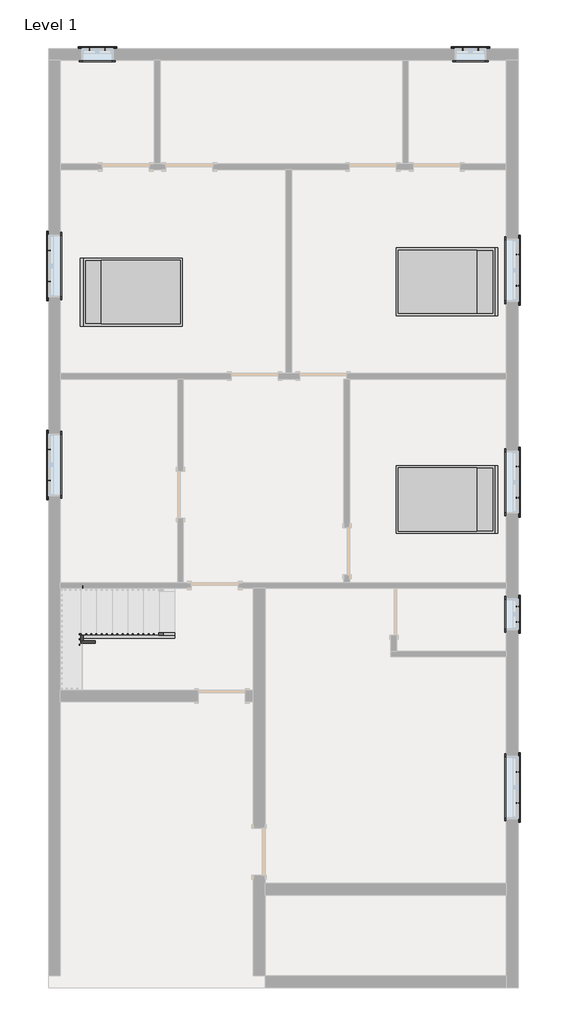
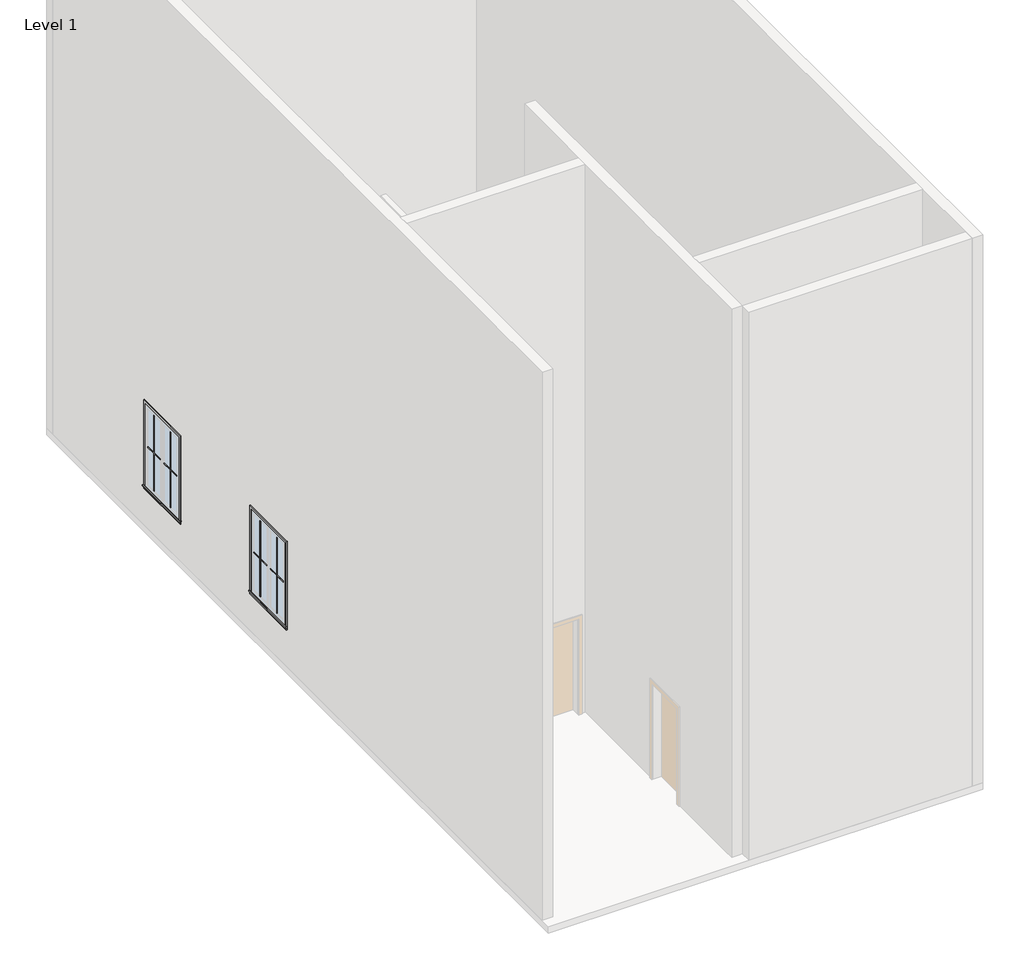
# One storey, part 2 of 2: 32 proxies, 6 members, 3 furniture elements, 1 railing.
"""IFC4 building model written with IfcOpenShell, lengths in millimetres."""

from ifc_helpers import new_model, si_unit, frame, origin, place, context, project, spatial, polyline, outline, extrude, faceted_brep, transform, mapped, element, save
from components import muntin_pattern_2x2_muntin_pattern_2x2_2b4d9f72, muntin_pattern_2x2_muntin_pattern_2x2_ef995ed3, muntin_pattern_2x2_muntin_pattern_2x2_53152e2c, muntin_pattern_2x2_muntin_pattern_2x2_e8f3e573, trim_window_exterior_flat_with_sill_b7e4d11c, trim_window_exterior_flat_with_sill_a665a915, trim_window_interior_flat_picture_frame_936b8d2a, trim_window_interior_flat_picture_frame_d485c387, bed_17739_bed_17739_15c61121

model = new_model("IFC4")

# Units and contexts
model_context = context("Model", 3, world=origin())
ifc_project = project(units=[si_unit("LENGTHUNIT", "METRE", prefix="MILLI")], contexts=[model_context])

# Site, building, storey
site = spatial("IfcSite", under=ifc_project)
building = spatial("IfcBuilding", under=site)
storey = spatial("IfcBuildingStorey", under=building, Name="Level 1", Elevation=0.0)

# Proxies
placement = place(None, origin())
muntin_pattern_2x2_muntin_pattern_2x2_shape = muntin_pattern_2x2_muntin_pattern_2x2_2b4d9f72(model_context)
element("IfcBuildingElementProxy", 1, Name="Muntin Pattern_2x2 : Muntin Pattern_2x2", ObjectType="Muntin Pattern_2x2 : Muntin Pattern_2x2", at=placement, inside=storey, context=model_context, shape_type="MappedRepresentation", body=[
    mapped(muntin_pattern_2x2_muntin_pattern_2x2_shape, transform((1279.525, 5811.8375, 984.25), x_axis=(0.0, 1.0, 0.0), y_axis=(-1.0, 0.0, 0.0), z_axis=(0.0, 0.0, 1.0))),
])
element("IfcBuildingElementProxy", 2, Name="Muntin Pattern_2x2 : Muntin Pattern_2x2", ObjectType="Muntin Pattern_2x2 : Muntin Pattern_2x2", at=placement, inside=storey, context=model_context, shape_type="MappedRepresentation", body=[
    mapped(muntin_pattern_2x2_muntin_pattern_2x2_shape, transform((1279.525, 9685.3375, 984.25), x_axis=(0.0, 1.0, 0.0), y_axis=(-1.0, 0.0, 0.0), z_axis=(0.0, 0.0, 1.0))),
])
element("IfcBuildingElementProxy", 3, Name="Muntin Pattern_2x2 : Muntin Pattern_2x2", ObjectType="Muntin Pattern_2x2 : Muntin Pattern_2x2", at=placement, inside=storey, context=model_context, shape_type="MappedRepresentation", body=[
    mapped(muntin_pattern_2x2_muntin_pattern_2x2_shape, transform((10404.475, 10209.2125, 984.25), x_axis=(0.0, -1.0, 0.0), y_axis=(1.0, 0.0, 0.0), z_axis=(0.0, 0.0, 1.0))),
])
element("IfcBuildingElementProxy", 4, Name="Muntin Pattern_2x2 : Muntin Pattern_2x2", ObjectType="Muntin Pattern_2x2 : Muntin Pattern_2x2", at=placement, inside=storey, context=model_context, shape_type="MappedRepresentation", body=[
    mapped(muntin_pattern_2x2_muntin_pattern_2x2_shape, transform((10404.475, 6081.7125, 984.25), x_axis=(0.0, -1.0, 0.0), y_axis=(1.0, 0.0, 0.0), z_axis=(0.0, 0.0, 1.0))),
])
element("IfcBuildingElementProxy", 5, Name="Muntin Pattern_2x2 : Muntin Pattern_2x2", ObjectType="Muntin Pattern_2x2 : Muntin Pattern_2x2", at=placement, inside=storey, context=model_context, shape_type="MappedRepresentation", body=[
    mapped(muntin_pattern_2x2_muntin_pattern_2x2_shape, transform((10404.475, 138.1125, 984.25), x_axis=(0.0, -1.0, 0.0), y_axis=(1.0, 0.0, 0.0), z_axis=(0.0, 0.0, 1.0))),
])
muntin_pattern_2x2_muntin_pattern_2x2_2_shape = muntin_pattern_2x2_muntin_pattern_2x2_ef995ed3(model_context)
element("IfcBuildingElementProxy", 6, Name="Muntin Pattern_2x2 : Muntin Pattern_2x2", ObjectType="Muntin Pattern_2x2 : Muntin Pattern_2x2", at=placement, inside=storey, context=model_context, shape_type="MappedRepresentation", body=[
    mapped(muntin_pattern_2x2_muntin_pattern_2x2_2_shape, transform((1279.525, 6418.2625, 984.25), x_axis=(0.0, -1.0, 0.0), y_axis=(1.0, 0.0, 0.0), z_axis=(0.0, 0.0, 1.0))),
])
element("IfcBuildingElementProxy", 7, Name="Muntin Pattern_2x2 : Muntin Pattern_2x2", ObjectType="Muntin Pattern_2x2 : Muntin Pattern_2x2", at=placement, inside=storey, context=model_context, shape_type="MappedRepresentation", body=[
    mapped(muntin_pattern_2x2_muntin_pattern_2x2_2_shape, transform((1279.525, 10291.7625, 984.25), x_axis=(0.0, -1.0, 0.0), y_axis=(1.0, 0.0, 0.0), z_axis=(0.0, 0.0, 1.0))),
])
element("IfcBuildingElementProxy", 8, Name="Muntin Pattern_2x2 : Muntin Pattern_2x2", ObjectType="Muntin Pattern_2x2 : Muntin Pattern_2x2", at=placement, inside=storey, context=model_context, shape_type="MappedRepresentation", body=[
    mapped(muntin_pattern_2x2_muntin_pattern_2x2_2_shape, transform((10404.475, 9602.7875, 984.25), x_axis=(0.0, 1.0, 0.0), y_axis=(-1.0, 0.0, 0.0), z_axis=(0.0, 0.0, 1.0))),
])
element("IfcBuildingElementProxy", 9, Name="Muntin Pattern_2x2 : Muntin Pattern_2x2", ObjectType="Muntin Pattern_2x2 : Muntin Pattern_2x2", at=placement, inside=storey, context=model_context, shape_type="MappedRepresentation", body=[
    mapped(muntin_pattern_2x2_muntin_pattern_2x2_2_shape, transform((10404.475, 5475.2875, 984.25), x_axis=(0.0, 1.0, 0.0), y_axis=(-1.0, 0.0, 0.0), z_axis=(0.0, 0.0, 1.0))),
])
element("IfcBuildingElementProxy", 10, Name="Muntin Pattern_2x2 : Muntin Pattern_2x2", ObjectType="Muntin Pattern_2x2 : Muntin Pattern_2x2", at=placement, inside=storey, context=model_context, shape_type="MappedRepresentation", body=[
    mapped(muntin_pattern_2x2_muntin_pattern_2x2_2_shape, transform((10404.475, -468.3125, 984.25), x_axis=(0.0, 1.0, 0.0), y_axis=(-1.0, 0.0, 0.0), z_axis=(0.0, 0.0, 1.0))),
])
muntin_pattern_2x2_muntin_pattern_2x2_3_shape = muntin_pattern_2x2_muntin_pattern_2x2_53152e2c(model_context)
element("IfcBuildingElementProxy", 11, Name="Muntin Pattern_2x2 : Muntin Pattern_2x2", ObjectType="Muntin Pattern_2x2 : Muntin Pattern_2x2", at=placement, inside=storey, context=model_context, shape_type="MappedRepresentation", body=[
    mapped(muntin_pattern_2x2_muntin_pattern_2x2_3_shape, transform((10404.475, 3357.5625, 984.25), x_axis=(0.0, -1.0, 0.0), y_axis=(1.0, 0.0, 0.0), z_axis=(0.0, 0.0, 1.0))),
])
element("IfcBuildingElementProxy", 12, Name="Muntin Pattern_2x2 : Muntin Pattern_2x2", ObjectType="Muntin Pattern_2x2 : Muntin Pattern_2x2", at=placement, inside=storey, context=model_context, shape_type="MappedRepresentation", body=[
    mapped(muntin_pattern_2x2_muntin_pattern_2x2_3_shape, transform((9336.0875, 14214.475, 984.25), x_axis=(1.0, 0.0, 0.0), y_axis=(0.0, 1.0, 0.0), z_axis=(0.0, 0.0, 1.0))),
])
element("IfcBuildingElementProxy", 13, Name="Muntin Pattern_2x2 : Muntin Pattern_2x2", ObjectType="Muntin Pattern_2x2 : Muntin Pattern_2x2", at=placement, inside=storey, context=model_context, shape_type="MappedRepresentation", body=[
    mapped(muntin_pattern_2x2_muntin_pattern_2x2_3_shape, transform((2071.6875, 14214.475, 984.25), x_axis=(1.0, 0.0, 0.0), y_axis=(0.0, 1.0, 0.0), z_axis=(0.0, 0.0, 1.0))),
])
muntin_pattern_2x2_muntin_pattern_2x2_4_shape = muntin_pattern_2x2_muntin_pattern_2x2_e8f3e573(model_context)
element("IfcBuildingElementProxy", 14, Name="Muntin Pattern_2x2 : Muntin Pattern_2x2", ObjectType="Muntin Pattern_2x2 : Muntin Pattern_2x2", at=placement, inside=storey, context=model_context, shape_type="MappedRepresentation", body=[
    mapped(muntin_pattern_2x2_muntin_pattern_2x2_4_shape, transform((10404.475, 3055.9375, 984.25), x_axis=(0.0, 1.0, 0.0), y_axis=(-1.0, 0.0, 0.0), z_axis=(0.0, 0.0, 1.0))),
])
element("IfcBuildingElementProxy", 15, Name="Muntin Pattern_2x2 : Muntin Pattern_2x2", ObjectType="Muntin Pattern_2x2 : Muntin Pattern_2x2", at=placement, inside=storey, context=model_context, shape_type="MappedRepresentation", body=[
    mapped(muntin_pattern_2x2_muntin_pattern_2x2_4_shape, transform((9637.7125, 14214.475, 984.25), x_axis=(-1.0, 0.0, 0.0), y_axis=(0.0, -1.0, 0.0), z_axis=(0.0, 0.0, 1.0))),
])
element("IfcBuildingElementProxy", 16, Name="Muntin Pattern_2x2 : Muntin Pattern_2x2", ObjectType="Muntin Pattern_2x2 : Muntin Pattern_2x2", at=placement, inside=storey, context=model_context, shape_type="MappedRepresentation", body=[
    mapped(muntin_pattern_2x2_muntin_pattern_2x2_4_shape, transform((2373.3125, 14214.475, 984.25), x_axis=(-1.0, 0.0, 0.0), y_axis=(0.0, -1.0, 0.0), z_axis=(0.0, 0.0, 1.0))),
])
trim_window_exterior_flat_with_sill_shape = trim_window_exterior_flat_with_sill_b7e4d11c(model_context)
element("IfcBuildingElementProxy", 17, Name="Trim-Window-Exterior-Flat : with Sill", ObjectType="Trim-Window-Exterior-Flat : with Sill", at=placement, inside=storey, context=model_context, shape_type="MappedRepresentation", body=[
    mapped(trim_window_exterior_flat_with_sill_shape, transform((1270.0, 6115.05, 2743.2), x_axis=(0.0, -1.0, 0.0), y_axis=(0.0, 0.0, 1.0), z_axis=(-1.0, 0.0, 0.0))),
])
element("IfcBuildingElementProxy", 18, Name="Trim-Window-Exterior-Flat : with Sill", ObjectType="Trim-Window-Exterior-Flat : with Sill", at=placement, inside=storey, context=model_context, shape_type="MappedRepresentation", body=[
    mapped(trim_window_exterior_flat_with_sill_shape, transform((1270.0, 9988.55, 2743.2), x_axis=(0.0, -1.0, 0.0), y_axis=(0.0, 0.0, 1.0), z_axis=(-1.0, 0.0, 0.0))),
])
element("IfcBuildingElementProxy", 19, Name="Trim-Window-Exterior-Flat : with Sill", ObjectType="Trim-Window-Exterior-Flat : with Sill", at=placement, inside=storey, context=model_context, shape_type="MappedRepresentation", body=[
    mapped(trim_window_exterior_flat_with_sill_shape, transform((10414.0, 9906.0, 2743.2), x_axis=(0.0, 1.0, 0.0), y_axis=(0.0, 0.0, 1.0), z_axis=(1.0, 0.0, 0.0))),
])
element("IfcBuildingElementProxy", 20, Name="Trim-Window-Exterior-Flat : with Sill", ObjectType="Trim-Window-Exterior-Flat : with Sill", at=placement, inside=storey, context=model_context, shape_type="MappedRepresentation", body=[
    mapped(trim_window_exterior_flat_with_sill_shape, transform((10414.0, 5778.5, 2743.2), x_axis=(0.0, 1.0, 0.0), y_axis=(0.0, 0.0, 1.0), z_axis=(1.0, 0.0, 0.0))),
])
element("IfcBuildingElementProxy", 21, Name="Trim-Window-Exterior-Flat : with Sill", ObjectType="Trim-Window-Exterior-Flat : with Sill", at=placement, inside=storey, context=model_context, shape_type="MappedRepresentation", body=[
    mapped(trim_window_exterior_flat_with_sill_shape, transform((10414.0, -165.1, 2743.2), x_axis=(0.0, 1.0, 0.0), y_axis=(0.0, 0.0, 1.0), z_axis=(1.0, 0.0, 0.0))),
])
trim_window_exterior_flat_with_sill_2_shape = trim_window_exterior_flat_with_sill_a665a915(model_context)
element("IfcBuildingElementProxy", 22, Name="Trim-Window-Exterior-Flat : with Sill", ObjectType="Trim-Window-Exterior-Flat : with Sill", at=placement, inside=storey, context=model_context, shape_type="MappedRepresentation", body=[
    mapped(trim_window_exterior_flat_with_sill_2_shape, transform((10414.0, 3206.75, 1828.8), x_axis=(0.0, 1.0, 0.0), y_axis=(0.0, 0.0, 1.0), z_axis=(1.0, 0.0, 0.0))),
])
element("IfcBuildingElementProxy", 23, Name="Trim-Window-Exterior-Flat : with Sill", ObjectType="Trim-Window-Exterior-Flat : with Sill", at=placement, inside=storey, context=model_context, shape_type="MappedRepresentation", body=[
    mapped(trim_window_exterior_flat_with_sill_2_shape, transform((9486.9, 14224.0, 1828.8), x_axis=(-1.0, 0.0, 0.0), y_axis=(0.0, 0.0, 1.0), z_axis=(0.0, 1.0, 0.0))),
])
element("IfcBuildingElementProxy", 24, Name="Trim-Window-Exterior-Flat : with Sill", ObjectType="Trim-Window-Exterior-Flat : with Sill", at=placement, inside=storey, context=model_context, shape_type="MappedRepresentation", body=[
    mapped(trim_window_exterior_flat_with_sill_2_shape, transform((2222.5, 14224.0, 1828.8), x_axis=(-1.0, 0.0, 0.0), y_axis=(0.0, 0.0, 1.0), z_axis=(0.0, 1.0, 0.0))),
])
trim_window_interior_flat_picture_frame_shape = trim_window_interior_flat_picture_frame_936b8d2a(model_context)
element("IfcBuildingElementProxy", 25, Name="Trim-Window-Interior-Flat : Picture Frame", ObjectType="Trim-Window-Interior-Flat : Picture Frame", at=placement, inside=storey, context=model_context, shape_type="MappedRepresentation", body=[
    mapped(trim_window_interior_flat_picture_frame_shape, transform((1498.6, 6115.05, 2743.2), x_axis=(0.0, 1.0, 0.0), y_axis=(0.0, 0.0, 1.0), z_axis=(1.0, 0.0, 0.0))),
])
element("IfcBuildingElementProxy", 26, Name="Trim-Window-Interior-Flat : Picture Frame", ObjectType="Trim-Window-Interior-Flat : Picture Frame", at=placement, inside=storey, context=model_context, shape_type="MappedRepresentation", body=[
    mapped(trim_window_interior_flat_picture_frame_shape, transform((1498.6, 9988.55, 2743.2), x_axis=(0.0, 1.0, 0.0), y_axis=(0.0, 0.0, 1.0), z_axis=(1.0, 0.0, 0.0))),
])
element("IfcBuildingElementProxy", 27, Name="Trim-Window-Interior-Flat : Picture Frame", ObjectType="Trim-Window-Interior-Flat : Picture Frame", at=placement, inside=storey, context=model_context, shape_type="MappedRepresentation", body=[
    mapped(trim_window_interior_flat_picture_frame_shape, transform((10185.4, 9906.0, 2743.2), x_axis=(0.0, -1.0, 0.0), y_axis=(0.0, 0.0, 1.0), z_axis=(-1.0, 0.0, 0.0))),
])
element("IfcBuildingElementProxy", 28, Name="Trim-Window-Interior-Flat : Picture Frame", ObjectType="Trim-Window-Interior-Flat : Picture Frame", at=placement, inside=storey, context=model_context, shape_type="MappedRepresentation", body=[
    mapped(trim_window_interior_flat_picture_frame_shape, transform((10185.4, 5778.5, 2743.2), x_axis=(0.0, -1.0, 0.0), y_axis=(0.0, 0.0, 1.0), z_axis=(-1.0, 0.0, 0.0))),
])
element("IfcBuildingElementProxy", 29, Name="Trim-Window-Interior-Flat : Picture Frame", ObjectType="Trim-Window-Interior-Flat : Picture Frame", at=placement, inside=storey, context=model_context, shape_type="MappedRepresentation", body=[
    mapped(trim_window_interior_flat_picture_frame_shape, transform((10185.4, -165.1, 2743.2), x_axis=(0.0, -1.0, 0.0), y_axis=(0.0, 0.0, 1.0), z_axis=(-1.0, 0.0, 0.0))),
])
trim_window_interior_flat_picture_frame_2_shape = trim_window_interior_flat_picture_frame_d485c387(model_context)
element("IfcBuildingElementProxy", 30, Name="Trim-Window-Interior-Flat : Picture Frame", ObjectType="Trim-Window-Interior-Flat : Picture Frame", at=placement, inside=storey, context=model_context, shape_type="MappedRepresentation", body=[
    mapped(trim_window_interior_flat_picture_frame_2_shape, transform((10185.4, 3206.75, 1828.8), x_axis=(0.0, -1.0, 0.0), y_axis=(0.0, 0.0, 1.0), z_axis=(-1.0, 0.0, 0.0))),
])
element("IfcBuildingElementProxy", 31, Name="Trim-Window-Interior-Flat : Picture Frame", ObjectType="Trim-Window-Interior-Flat : Picture Frame", at=placement, inside=storey, context=model_context, shape_type="MappedRepresentation", body=[
    mapped(trim_window_interior_flat_picture_frame_2_shape, transform((9486.9, 13995.4, 1828.8), x_axis=(1.0, 0.0, 0.0), y_axis=(0.0, 0.0, 1.0), z_axis=(0.0, -1.0, 0.0))),
])
element("IfcBuildingElementProxy", 32, Name="Trim-Window-Interior-Flat : Picture Frame", ObjectType="Trim-Window-Interior-Flat : Picture Frame", at=placement, inside=storey, context=model_context, shape_type="MappedRepresentation", body=[
    mapped(trim_window_interior_flat_picture_frame_2_shape, transform((2222.5, 13995.4, 1828.8), x_axis=(1.0, 0.0, 0.0), y_axis=(0.0, 0.0, 1.0), z_axis=(0.0, -1.0, 0.0))),
])

# Furniture
bed_17739_bed_17739_shape = bed_17739_bed_17739_15c61121(model_context)
element("IfcFurniture", 33, ObjectType="Bed_17739 : Bed_17739", at=placement, inside=storey, context=model_context, shape_type="MappedRepresentation", body=[
    mapped(bed_17739_bed_17739_shape, transform((2908.3, 9480.55, 0.0), x_axis=(0.0, 1.0, 0.0), y_axis=(-1.0, 0.0, 0.0), z_axis=(0.0, 0.0, 1.0))),
])
element("IfcFurniture", 34, ObjectType="Bed_17739 : Bed_17739", at=placement, inside=storey, context=model_context, shape_type="MappedRepresentation", body=[
    mapped(bed_17739_bed_17739_shape, transform((9004.792661, 9680.2142579, 0.0), x_axis=(0.0, -1.0, 0.0), y_axis=(1.0, 0.0, 0.0), z_axis=(0.0, 0.0, 1.0))),
])
element("IfcFurniture", 35, ObjectType="Bed_17739 : Bed_17739", at=placement, inside=storey, context=model_context, shape_type="MappedRepresentation", body=[
    mapped(bed_17739_bed_17739_shape, transform((9004.792661, 5441.95, 0.0), x_axis=(0.0, -1.0, 0.0), y_axis=(1.0, 0.0, 0.0), z_axis=(0.0, 0.0, 1.0))),
])

# Members
element("IfcMember", 36, ObjectType="Stringer - 2\" Width", at=placement, inside=storey, context=model_context, shape_type="SweptSolid", body=[
    extrude(outline(polyline([(0.0, 3727.9146873), (207.5983948, 3727.9146873), (1195.3761726, 1949.9146873), (846.6974984, 1949.9146873), (0.0, 3473.9701845), (0.0, 3727.9146873)])), frame((0.0, 2743.2, 0.0), z_axis=(0.0, 1.0, 0.0), x_axis=(0.0, 0.0, 1.0)), (0.0, 0.0, 1.0), 50.8),
])
element("IfcMember", 37, ObjectType="Stringer - 2\" Width", at=placement, inside=storey, context=model_context, shape_type="SweptSolid", body=[
    extrude(outline(polyline([(1899.1146873, 2794.0), (1949.9146873, 2794.0), (1949.9146873, 2692.4), (1899.1146873, 2692.4), (1899.1146873, 2794.0)])), frame((0.0, 0.0, 956.7333333), z_axis=(0.0, 0.0, 1.0), x_axis=(1.0, 0.0, 0.0)), (0.0, 0.0, 1.0), 304.8),
])
element("IfcMember", 38, ObjectType="Stringer - 2\" Width", at=placement, inside=storey, context=model_context, shape_type="SweptSolid", body=[
    extrude(outline(polyline([(1392.9317281, 1899.1146873), (1044.253054, 1899.1146873), (2060.253054, 3727.9146873), (2408.9317281, 3727.9146873), (1392.9317281, 1899.1146873)])), frame((0.0, 2641.6, 0.0), z_axis=(0.0, 1.0, 0.0), x_axis=(0.0, 0.0, 1.0)), (0.0, 0.0, 1.0), 50.8),
])
element("IfcMember", 39, ObjectType="Stringer - 2\" Width", at=placement, inside=storey, context=model_context, shape_type="SweptSolid", body=[
    extrude(outline(polyline([(0.0, 3727.9146873), (207.5983948, 3727.9146873), (1261.5333333, 1830.8317979), (1261.5333333, 1498.6), (1097.4278803, 1498.6), (0.0, 3473.9701845), (0.0, 3727.9146873)])), frame((0.0, 3708.4, 0.0), z_axis=(0.0, 1.0, 0.0), x_axis=(0.0, 0.0, 1.0)), (0.0, 0.0, 1.0), 50.8),
])
element("IfcMember", 40, ObjectType="Stringer - 2\" Width", at=placement, inside=storey, context=model_context, shape_type="SweptSolid", body=[
    extrude(outline(polyline([(1447.8, 3759.2), (1498.6, 3759.2), (1498.6, 1727.2), (1447.8, 1727.2), (1447.8, 3759.2)])), frame((0.0, 0.0, 956.7333333), z_axis=(0.0, 0.0, 1.0), x_axis=(1.0, 0.0, 0.0)), (0.0, 0.0, 1.0), 304.8),
])
element("IfcMember", 41, ObjectType="Stringer - 2\" Width", at=placement, inside=storey, context=model_context, shape_type="SweptSolid", body=[
    extrude(outline(polyline([(1142.2013463, 1447.8), (956.7333333, 1447.8), (956.7333333, 1741.5791901), (2060.253054, 3727.9146873), (2408.9317281, 3727.9146873), (1142.2013463, 1447.8)])), frame((0.0, 1676.4, 0.0), z_axis=(0.0, 1.0, 0.0), x_axis=(0.0, 0.0, 1.0)), (0.0, 0.0, 1.0), 50.8),
])

# Railing
element("IfcRailing", 42, ObjectType="Handrail - Rectangular", at=placement, inside=storey, context=model_context, shape_type="SolidModel", body=[
    faceted_brep([(3727.9146873, 2794.0, 1083.7333333), (3727.9146873, 2794.0, 1025.620221), (3727.9146873, 2844.8, 1025.620221), (3727.9146873, 2844.8, 1083.7333333), (1975.3146873, 2794.0, 2057.4), (1924.5146873, 2794.0, 2027.5091099), (1924.5146873, 2844.8, 2027.5091099), (1975.3146873, 2844.8, 2057.4), (1975.3146873, 2794.0, 2099.7333333), (1924.5146873, 2794.0, 2048.9333333), (1924.5146873, 2844.8, 2048.9333333), (1975.3146873, 2844.8, 2099.7333333), (1899.1146873, 2794.0, 2099.7333333), (1899.1146873, 2794.0, 2048.9333333), (1848.3146873, 2844.8, 2048.9333333), (1848.3146873, 2844.8, 2099.7333333), (1899.1146873, 2717.8, 2099.7333333), (1899.1146873, 2667.0, 2048.9333333), (1848.3146873, 2667.0, 2048.9333333), (1848.3146873, 2717.8, 2099.7333333), (1899.1146873, 2717.8, 2311.4), (1899.1146873, 2667.0, 2260.6), (1848.3146873, 2667.0, 2260.6), (1848.3146873, 2717.8, 2311.4), (1899.1146873, 2641.6, 2311.4), (1899.1146873, 2641.6, 2260.6), (1848.3146873, 2590.8, 2260.6), (1848.3146873, 2590.8, 2311.4), (1975.3146873, 2641.6, 2311.4), (1988.4782895, 2641.6, 2260.6), (1988.4782895, 2590.8, 2260.6), (1975.3146873, 2590.8, 2311.4), (3727.9146873, 2641.6, 3285.0666667), (3727.9146873, 2590.8, 3285.0666667), (3727.9146873, 2590.8, 3226.9535543), (3727.9146873, 2641.6, 3226.9535543)], [[[0, 1, 2, 3]], [[1, 0, 4, 5]], [[2, 1, 5, 6]], [[3, 2, 6, 7]], [[0, 3, 7, 4]], [[5, 4, 8, 9]], [[6, 5, 9, 10]], [[7, 6, 10, 11]], [[4, 7, 11, 8]], [[9, 8, 12, 13]], [[10, 9, 13, 14]], [[11, 10, 14, 15]], [[8, 11, 15, 12]], [[13, 12, 16, 17]], [[14, 13, 17, 18]], [[15, 14, 18, 19]], [[12, 15, 19, 16]], [[17, 16, 20, 21]], [[18, 17, 21, 22]], [[19, 18, 22, 23]], [[16, 19, 23, 20]], [[21, 20, 24, 25]], [[22, 21, 25, 26]], [[23, 22, 26, 27]], [[20, 23, 27, 24]], [[25, 24, 28, 29]], [[26, 25, 29, 30]], [[27, 26, 30, 31]], [[24, 27, 31, 28]], [[32, 33, 34, 35]], [[29, 28, 32, 35]], [[30, 29, 35, 34]], [[31, 30, 34, 33]], [[28, 31, 33, 32]]]),
    extrude(outline(polyline([(3207.5507765, 3692.9896873), (2201.3333333, 3692.9896873), (2201.3333333, 3712.0396873), (3218.1341099, 3712.0396873), (3207.5507765, 3692.9896873)])), frame((0.0, 2606.675, 0.0), z_axis=(0.0, 1.0, 0.0), x_axis=(0.0, 0.0, 1.0)), (0.0, 0.0, 1.0), 19.05),
    extrude(outline(polyline([(3151.1063321, 3591.3896873), (2201.3333333, 3591.3896873), (2201.3333333, 3610.4396873), (3161.6896654, 3610.4396873), (3151.1063321, 3591.3896873)])), frame((0.0, 2606.675, 0.0), z_axis=(0.0, 1.0, 0.0), x_axis=(0.0, 0.0, 1.0)), (0.0, 0.0, 1.0), 19.05),
    extrude(outline(polyline([(3094.6618876, 3489.7896873), (2201.3333333, 3489.7896873), (2201.3333333, 3508.8396873), (3105.245221, 3508.8396873), (3094.6618876, 3489.7896873)])), frame((0.0, 2606.675, 0.0), z_axis=(0.0, 1.0, 0.0), x_axis=(0.0, 0.0, 1.0)), (0.0, 0.0, 1.0), 19.05),
    extrude(outline(polyline([(3038.2174432, 3388.1896873), (2032.0, 3388.1896873), (2032.0, 3407.2396873), (3048.8007765, 3407.2396873), (3038.2174432, 3388.1896873)])), frame((0.0, 2606.675, 0.0), z_axis=(0.0, 1.0, 0.0), x_axis=(0.0, 0.0, 1.0)), (0.0, 0.0, 1.0), 19.05),
    extrude(outline(polyline([(2981.7729988, 3286.5896873), (2032.0, 3286.5896873), (2032.0, 3305.6396873), (2992.3563321, 3305.6396873), (2981.7729988, 3286.5896873)])), frame((0.0, 2606.675, 0.0), z_axis=(0.0, 1.0, 0.0), x_axis=(0.0, 0.0, 1.0)), (0.0, 0.0, 1.0), 19.05),
    extrude(outline(polyline([(2925.3285543, 3184.9896873), (2032.0, 3184.9896873), (2032.0, 3204.0396873), (2935.9118876, 3204.0396873), (2925.3285543, 3184.9896873)])), frame((0.0, 2606.675, 0.0), z_axis=(0.0, 1.0, 0.0), x_axis=(0.0, 0.0, 1.0)), (0.0, 0.0, 1.0), 19.05),
    extrude(outline(polyline([(2868.8841099, 3083.3896873), (1862.6666667, 3083.3896873), (1862.6666667, 3102.4396873), (2879.4674432, 3102.4396873), (2868.8841099, 3083.3896873)])), frame((0.0, 2606.675, 0.0), z_axis=(0.0, 1.0, 0.0), x_axis=(0.0, 0.0, 1.0)), (0.0, 0.0, 1.0), 19.05),
    extrude(outline(polyline([(2812.4396654, 2981.7896873), (1862.6666667, 2981.7896873), (1862.6666667, 3000.8396873), (2823.0229988, 3000.8396873), (2812.4396654, 2981.7896873)])), frame((0.0, 2606.675, 0.0), z_axis=(0.0, 1.0, 0.0), x_axis=(0.0, 0.0, 1.0)), (0.0, 0.0, 1.0), 19.05),
    extrude(outline(polyline([(2755.995221, 2880.1896873), (1862.6666667, 2880.1896873), (1862.6666667, 2899.2396873), (2766.5785543, 2899.2396873), (2755.995221, 2880.1896873)])), frame((0.0, 2606.675, 0.0), z_axis=(0.0, 1.0, 0.0), x_axis=(0.0, 0.0, 1.0)), (0.0, 0.0, 1.0), 19.05),
    extrude(outline(polyline([(2699.5507765, 2778.5896873), (1693.3333333, 2778.5896873), (1693.3333333, 2797.6396873), (2710.1341099, 2797.6396873), (2699.5507765, 2778.5896873)])), frame((0.0, 2606.675, 0.0), z_axis=(0.0, 1.0, 0.0), x_axis=(0.0, 0.0, 1.0)), (0.0, 0.0, 1.0), 19.05),
    extrude(outline(polyline([(2643.1063321, 2676.9896873), (1693.3333333, 2676.9896873), (1693.3333333, 2696.0396873), (2653.6896654, 2696.0396873), (2643.1063321, 2676.9896873)])), frame((0.0, 2606.675, 0.0), z_axis=(0.0, 1.0, 0.0), x_axis=(0.0, 0.0, 1.0)), (0.0, 0.0, 1.0), 19.05),
    extrude(outline(polyline([(2586.6618876, 2575.3896873), (1693.3333333, 2575.3896873), (1693.3333333, 2594.4396873), (2597.245221, 2594.4396873), (2586.6618876, 2575.3896873)])), frame((0.0, 2606.675, 0.0), z_axis=(0.0, 1.0, 0.0), x_axis=(0.0, 0.0, 1.0)), (0.0, 0.0, 1.0), 19.05),
    extrude(outline(polyline([(2530.2174432, 2473.7896873), (1524.0, 2473.7896873), (1524.0, 2492.8396873), (2540.8007765, 2492.8396873), (2530.2174432, 2473.7896873)])), frame((0.0, 2606.675, 0.0), z_axis=(0.0, 1.0, 0.0), x_axis=(0.0, 0.0, 1.0)), (0.0, 0.0, 1.0), 19.05),
    extrude(outline(polyline([(2473.7729988, 2372.1896873), (1524.0, 2372.1896873), (1524.0, 2391.2396873), (2484.3563321, 2391.2396873), (2473.7729988, 2372.1896873)])), frame((0.0, 2606.675, 0.0), z_axis=(0.0, 1.0, 0.0), x_axis=(0.0, 0.0, 1.0)), (0.0, 0.0, 1.0), 19.05),
    extrude(outline(polyline([(2417.3285543, 2270.5896873), (1524.0, 2270.5896873), (1524.0, 2289.6396873), (2427.9118876, 2289.6396873), (2417.3285543, 2270.5896873)])), frame((0.0, 2606.675, 0.0), z_axis=(0.0, 1.0, 0.0), x_axis=(0.0, 0.0, 1.0)), (0.0, 0.0, 1.0), 19.05),
    extrude(outline(polyline([(2360.8841099, 2168.9896873), (1354.6666667, 2168.9896873), (1354.6666667, 2188.0396873), (2371.4674432, 2188.0396873), (2360.8841099, 2168.9896873)])), frame((0.0, 2606.675, 0.0), z_axis=(0.0, 1.0, 0.0), x_axis=(0.0, 0.0, 1.0)), (0.0, 0.0, 1.0), 19.05),
    extrude(outline(polyline([(2304.4396654, 2067.3896873), (1354.6666667, 2067.3896873), (1354.6666667, 2086.4396873), (2315.0229988, 2086.4396873), (2304.4396654, 2067.3896873)])), frame((0.0, 2606.675, 0.0), z_axis=(0.0, 1.0, 0.0), x_axis=(0.0, 0.0, 1.0)), (0.0, 0.0, 1.0), 19.05),
    extrude(outline(polyline([(2247.995221, 1965.7896873), (1354.6666667, 1965.7896873), (1354.6666667, 1984.8396873), (2258.5785543, 1984.8396873), (2247.995221, 1965.7896873)])), frame((0.0, 2606.675, 0.0), z_axis=(0.0, 1.0, 0.0), x_axis=(0.0, 0.0, 1.0)), (0.0, 0.0, 1.0), 19.05),
    extrude(outline(polyline([(1883.2396873, 2727.325), (1883.2396873, 2708.275), (1864.1896873, 2708.275), (1864.1896873, 2727.325), (1883.2396873, 2727.325)])), frame((0.0, 0.0, 1185.3333333), z_axis=(0.0, 0.0, 1.0), x_axis=(1.0, 0.0, 0.0)), (0.0, 0.0, 1.0), 863.6),
    extrude(outline(polyline([(1908.6396873, 2809.875), (1889.5896873, 2809.875), (1889.5896873, 2828.925), (1908.6396873, 2828.925), (1908.6396873, 2809.875)])), frame((0.0, 0.0, 1185.3333333), z_axis=(0.0, 0.0, 1.0), x_axis=(1.0, 0.0, 0.0)), (0.0, 0.0, 1.0), 863.6),
    extrude(outline(polyline([(1990.4674432, 1991.1896873), (1016.0, 1991.1896873), (1016.0, 2010.2396873), (1979.8841099, 2010.2396873), (1990.4674432, 1991.1896873)])), frame((0.0, 2809.875, 0.0), z_axis=(0.0, 1.0, 0.0), x_axis=(0.0, 0.0, 1.0)), (0.0, 0.0, 1.0), 19.05),
    extrude(outline(polyline([(1934.0229988, 2092.7896873), (1016.0, 2092.7896873), (1016.0, 2111.8396873), (1923.4396654, 2111.8396873), (1934.0229988, 2092.7896873)])), frame((0.0, 2809.875, 0.0), z_axis=(0.0, 1.0, 0.0), x_axis=(0.0, 0.0, 1.0)), (0.0, 0.0, 1.0), 19.05),
    extrude(outline(polyline([(1877.5785543, 2194.3896873), (1016.0, 2194.3896873), (1016.0, 2213.4396873), (1866.995221, 2213.4396873), (1877.5785543, 2194.3896873)])), frame((0.0, 2809.875, 0.0), z_axis=(0.0, 1.0, 0.0), x_axis=(0.0, 0.0, 1.0)), (0.0, 0.0, 1.0), 19.05),
    extrude(outline(polyline([(1821.1341099, 2295.9896873), (846.6666667, 2295.9896873), (846.6666667, 2315.0396873), (1810.5507765, 2315.0396873), (1821.1341099, 2295.9896873)])), frame((0.0, 2809.875, 0.0), z_axis=(0.0, 1.0, 0.0), x_axis=(0.0, 0.0, 1.0)), (0.0, 0.0, 1.0), 19.05),
    extrude(outline(polyline([(1764.6896654, 2397.5896873), (846.6666667, 2397.5896873), (846.6666667, 2416.6396873), (1754.1063321, 2416.6396873), (1764.6896654, 2397.5896873)])), frame((0.0, 2809.875, 0.0), z_axis=(0.0, 1.0, 0.0), x_axis=(0.0, 0.0, 1.0)), (0.0, 0.0, 1.0), 19.05),
    extrude(outline(polyline([(1708.245221, 2499.1896873), (846.6666667, 2499.1896873), (846.6666667, 2518.2396873), (1697.6618876, 2518.2396873), (1708.245221, 2499.1896873)])), frame((0.0, 2809.875, 0.0), z_axis=(0.0, 1.0, 0.0), x_axis=(0.0, 0.0, 1.0)), (0.0, 0.0, 1.0), 19.05),
    extrude(outline(polyline([(1651.8007765, 2600.7896873), (677.3333333, 2600.7896873), (677.3333333, 2619.8396873), (1641.2174432, 2619.8396873), (1651.8007765, 2600.7896873)])), frame((0.0, 2809.875, 0.0), z_axis=(0.0, 1.0, 0.0), x_axis=(0.0, 0.0, 1.0)), (0.0, 0.0, 1.0), 19.05),
    extrude(outline(polyline([(1595.3563321, 2702.3896873), (677.3333333, 2702.3896873), (677.3333333, 2721.4396873), (1584.7729988, 2721.4396873), (1595.3563321, 2702.3896873)])), frame((0.0, 2809.875, 0.0), z_axis=(0.0, 1.0, 0.0), x_axis=(0.0, 0.0, 1.0)), (0.0, 0.0, 1.0), 19.05),
    extrude(outline(polyline([(1538.9118876, 2803.9896873), (677.3333333, 2803.9896873), (677.3333333, 2823.0396873), (1528.3285543, 2823.0396873), (1538.9118876, 2803.9896873)])), frame((0.0, 2809.875, 0.0), z_axis=(0.0, 1.0, 0.0), x_axis=(0.0, 0.0, 1.0)), (0.0, 0.0, 1.0), 19.05),
    extrude(outline(polyline([(1482.4674432, 2905.5896873), (508.0, 2905.5896873), (508.0, 2924.6396873), (1471.8841099, 2924.6396873), (1482.4674432, 2905.5896873)])), frame((0.0, 2809.875, 0.0), z_axis=(0.0, 1.0, 0.0), x_axis=(0.0, 0.0, 1.0)), (0.0, 0.0, 1.0), 19.05),
    extrude(outline(polyline([(1426.0229988, 3007.1896873), (508.0, 3007.1896873), (508.0, 3026.2396873), (1415.4396654, 3026.2396873), (1426.0229988, 3007.1896873)])), frame((0.0, 2809.875, 0.0), z_axis=(0.0, 1.0, 0.0), x_axis=(0.0, 0.0, 1.0)), (0.0, 0.0, 1.0), 19.05),
    extrude(outline(polyline([(1369.5785543, 3108.7896873), (508.0, 3108.7896873), (508.0, 3127.8396873), (1358.995221, 3127.8396873), (1369.5785543, 3108.7896873)])), frame((0.0, 2809.875, 0.0), z_axis=(0.0, 1.0, 0.0), x_axis=(0.0, 0.0, 1.0)), (0.0, 0.0, 1.0), 19.05),
    extrude(outline(polyline([(1313.1341099, 3210.3896873), (338.6666667, 3210.3896873), (338.6666667, 3229.4396873), (1302.5507765, 3229.4396873), (1313.1341099, 3210.3896873)])), frame((0.0, 2809.875, 0.0), z_axis=(0.0, 1.0, 0.0), x_axis=(0.0, 0.0, 1.0)), (0.0, 0.0, 1.0), 19.05),
    extrude(outline(polyline([(1256.6896654, 3311.9896873), (338.6666667, 3311.9896873), (338.6666667, 3331.0396873), (1246.1063321, 3331.0396873), (1256.6896654, 3311.9896873)])), frame((0.0, 2809.875, 0.0), z_axis=(0.0, 1.0, 0.0), x_axis=(0.0, 0.0, 1.0)), (0.0, 0.0, 1.0), 19.05),
    extrude(outline(polyline([(1200.245221, 3413.5896873), (338.6666667, 3413.5896873), (338.6666667, 3432.6396873), (1189.6618876, 3432.6396873), (1200.245221, 3413.5896873)])), frame((0.0, 2809.875, 0.0), z_axis=(0.0, 1.0, 0.0), x_axis=(0.0, 0.0, 1.0)), (0.0, 0.0, 1.0), 19.05),
    extrude(outline(polyline([(1143.8007765, 3515.1896873), (169.3333333, 3515.1896873), (169.3333333, 3534.2396873), (1133.2174432, 3534.2396873), (1143.8007765, 3515.1896873)])), frame((0.0, 2809.875, 0.0), z_axis=(0.0, 1.0, 0.0), x_axis=(0.0, 0.0, 1.0)), (0.0, 0.0, 1.0), 19.05),
    extrude(outline(polyline([(1087.3563321, 3616.7896873), (169.3333333, 3616.7896873), (169.3333333, 3635.8396873), (1076.7729988, 3635.8396873), (1087.3563321, 3616.7896873)])), frame((0.0, 2809.875, 0.0), z_axis=(0.0, 1.0, 0.0), x_axis=(0.0, 0.0, 1.0)), (0.0, 0.0, 1.0), 19.05),
    extrude(outline(polyline([(1883.2396873, 2625.725), (1883.2396873, 2606.675), (1864.1896873, 2606.675), (1864.1896873, 2625.725), (1883.2396873, 2625.725)])), frame((0.0, 0.0, 1185.3333333), z_axis=(0.0, 0.0, 1.0), x_axis=(1.0, 0.0, 0.0)), (0.0, 0.0, 1.0), 1075.2666667),
    extrude(outline(polyline([(1883.2396873, 2809.875), (1864.1896873, 2809.875), (1864.1896873, 2828.925), (1883.2396873, 2828.925), (1883.2396873, 2809.875)])), frame((0.0, 0.0, 1185.3333333), z_axis=(0.0, 0.0, 1.0), x_axis=(1.0, 0.0, 0.0)), (0.0, 0.0, 1.0), 863.6),
    extrude(outline(polyline([(3216.370221, 3708.8646873), (2201.3333333, 3708.8646873), (2201.3333333, 3727.9146873), (3226.9535543, 3727.9146873), (3216.370221, 3708.8646873)])), frame((0.0, 2606.675, 0.0), z_axis=(0.0, 1.0, 0.0), x_axis=(0.0, 0.0, 1.0)), (0.0, 0.0, 1.0), 19.05),
    extrude(outline(polyline([(1036.2035543, 3708.8646873), (169.3333333, 3708.8646873), (169.3333333, 3727.9146873), (1025.620221, 3727.9146873), (1036.2035543, 3708.8646873)])), frame((0.0, 2809.875, 0.0), z_axis=(0.0, 1.0, 0.0), x_axis=(0.0, 0.0, 1.0)), (0.0, 0.0, 1.0), 19.05),
])

save(model, "model.ifc")

# Revit data of these elements
# Type "Muntin Pattern_2x2 : Muntin Pattern_2x2"
#   Width [instance default] = 4' - 0"
#   Thickness = 0' - 0 1/2"
#   Height [instance default] = 4' - 0"
#   Distance = 0' - 0 3/4"
#   Interior Material [instance default] = none
#   Exterior Material [instance default] = none
#   Default Elevation = 0
# Type "Trim-Window-Exterior-Flat : with Sill"
#   Trim Width = 0' - 2 1/4"
#   Trim Thickness_Picture Frame = 0' - 1 1/4"
#   Trim Thickness_with Sill = 0' - 0 3/4"
#   Sill Thickness = 0' - 1 1/4"
#   Opening Width [instance default] = 2' - 0"
#   Opening Height [instance default] = 3' - 0"
#   Default Elevation = 4' - 0"
#   Sill = yes
#   Picture Frame = no
#   Trim Material [instance default] = none
# Type "Trim-Window-Interior-Flat : Picture Frame"
#   Trim Thickness_Picture Frame = 0' - 1 1/4"
#   Trim Width = 0' - 2 1/4"
#   Trim Thickness_with Sill = 0' - 0 3/4"
#   Sill Thickness = 0' - 1 1/4"
#   Opening Width [instance default] = 2' - 0"
#   Opening Height [instance default] = 3' - 0"
#   Default Elevation = 4' - 0"
#   Sill = no
#   Picture Frame = yes
#   Trim Material [instance default] = none
# Type "Bed_17739 : Bed_17739"
#   Default Elevation = 0
# Type "Handrail - Rectangular"
#   Assembly Code = "C2010400"
#   built-in parameter 1008612 = 0.0416667 (stored number, unit not read)
#   built-in parameter 1008611 = 0.0416667 (stored number, unit not read)
#   built-in parameter 1008609 = 0.333333 (stored number, unit not read)
#   built-in parameter 1008604 = 0.166667 (stored number, unit not read)
#   built-in parameter 1008603 = 0.166667 (stored number, unit not read)
#   Railing Height = 3' - 0"
#   built-in parameter 1008630 = 2
#   built-in parameter 1008610 = 2
#   built-in parameter 1008618 = Baluster - Square : 3/4"
# Elements 1, 2, 3, 4, 5, 6, 7, 8, 9, 10 (IfcBuildingElementProxy, "Muntin Pattern_2x2 : Muntin Pattern_2x2")
#   Width = 1' - 6 5/8"
#   Height = 5' - 6 1/2"
#   Interior Material = Wood - Stained
#   Exterior Material = Clad - White
#   Phase Created = New Construction
#   Materials on its faces: "Clad - White", "Wood - Stained"
# Elements 11, 12, 13, 14, 15, 16 (IfcBuildingElementProxy, "Muntin Pattern_2x2 : Muntin Pattern_2x2")
#   Width = 0' - 6 5/8"
#   Height = 2' - 6 1/2"
#   Interior Material = Wood - Stained
#   Exterior Material = Clad - White
#   Phase Created = New Construction
#   Materials on its faces: "Clad - White", "Wood - Stained"
# Elements 17, 18, 19, 20, 21 (IfcBuildingElementProxy, "Trim-Window-Exterior-Flat : with Sill")
#   Opening Width = 4' - 0"
#   Opening Height = 6' - 0"
#   Trim Material = Clad - White
#   Phase Created = New Construction
#   Materials on its faces: "Clad - White"
# Elements 22, 23, 24 (IfcBuildingElementProxy, "Trim-Window-Exterior-Flat : with Sill")
#   Opening Width = 2' - 0"
#   Opening Height = 3' - 0"
#   Trim Material = Clad - White
#   Phase Created = New Construction
#   Materials on its faces: "Clad - White"
# Elements 25, 26, 27, 28, 29 (IfcBuildingElementProxy, "Trim-Window-Interior-Flat : Picture Frame")
#   Opening Width = 4' - 0"
#   Opening Height = 6' - 0"
#   Trim Material = Wood - Stained
#   Phase Created = New Construction
#   Materials on its faces: "Wood - Stained"
# Elements 30, 31, 32 (IfcBuildingElementProxy, "Trim-Window-Interior-Flat : Picture Frame")
#   Opening Width = 2' - 0"
#   Opening Height = 3' - 0"
#   Trim Material = Wood - Stained
#   Phase Created = New Construction
#   Materials on its faces: "Wood - Stained"
# Elements 33, 34, 35 (IfcFurniture, "Bed_17739 : Bed_17739")
#   Phase Created = New Construction
#   Materials on its faces: "legs", "sheets", "bed frame", "Blanket"
# Elements 36, 37, 38, 39, 40, 41 (IfcMember, "Stringer - 2\" Width")
#   Phase Created = New Construction
# Element 42 (IfcRailing, "Handrail - Rectangular")
#   Phase Created = New Construction
# Materials
#   "Clad - White": class "Wood", colour RGB 242 242 238, transparency 0, Cost = 0
#   "Wood - Stained": class "Wood", colour RGB 224 178 126, transparency 0, Cost = 0
#   "legs": colour RGB 90 73 37, transparency 0, Cost = 0
#   "sheets": colour RGB 200 195 176, transparency 0, Cost = 0
#   "bed frame": colour RGB 90 73 37, transparency 0, Cost = 0
#   "Blanket": class "System", colour RGB 59 0 1, transparency 0, Cost = 0
